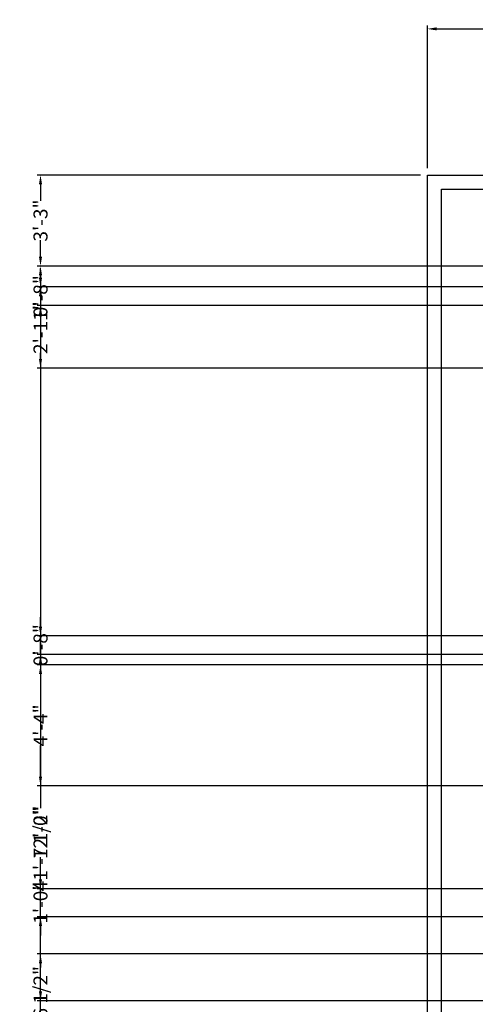
# Model space of a CAD drawing. Units: inches. Extents: x 6704 to 7574, y 11759 to 12617.
# Tile 3 of 8: x 6704 to 6900, y 12195 to 12617. Entities that reach past the tile are written whole.
import ezdxf

# ---------------------------------------------------------------- set-up
doc = ezdxf.new("R2010")
doc.units = ezdxf.units.IN
doc.header["$MEASUREMENT"] = 0
doc.layers.add('C-PROP', color=7, linetype='Continuous', lineweight=30)
doc.layers.add('YQ_DIM', color=3, linetype='Continuous', lineweight=18)
doc.styles.get("Standard").update_dxf_attribs({"font": 'arial.ttf'})
doc.dimstyles.new('yqi0', dxfattribs={"dimscale": 0, "dimtxt": 6, "dimasz": 4, "dimexe": 1.5, "dimexo": 3, "dimgap": 0.5, "dimtad": 0, "dimdsep": 46, "dimlunit": 4, "dimtxsty": 'Standard', "dimcen": 0, "dimclrd": 256, "dimclre": 256, "dimclrt": 7, "dimadec": 1, "dimazin": 2, "dimtfac": 1, "dimtix": 1, "dimtmove": 2, "dimatfit": 2, "dimfxl": 1, "dimtolj": 1, "dimtzin": 0, "dimarcsym": 0})

# ---------------------------------------------------------------- blocks, each defined once
blk = doc.blocks.new('*D2')
at = {"layer": 'Defpoints', "color": 0, "transparency": 16777216}
for p in [(7311.07, 12612.93), (6879.07, 12550.26), (7311.07, 12550.26)]:
    blk.add_point(p, dxfattribs=at)
at = {"layer": 'YQ_DIM', "color": 0, "lineweight": -2, "transparency": 16777216}
for p, q in [((6879.07, 12553.26), (6879.07, 12614.43)), ((7311.07, 12553.26), (7311.07, 12614.43)), ((6883.07, 12612.93), (7089.48, 12612.93)), ((7307.07, 12612.93), (7100.66, 12612.93))]:
    blk.add_line(p, q, dxfattribs=at)
at = {"layer": 'YQ_DIM', "color": 0, "transparency": 16777216}
for points in [[(6883.07, 12613.6), (6883.07, 12612.27), (6879.07, 12612.93)], [(7307.07, 12613.6), (7307.07, 12612.27), (7311.07, 12612.93)]]:
    blk.add_solid(points, dxfattribs=at)
at = {"layer": 'YQ_DIM', "color": 0, "transparency": 16777216, "insert": (7095.07, 12612.93), "char_height": 6, "attachment_point": 5}
blk.add_mtext("\\A1;36'", dxfattribs=at)
blk = doc.blocks.new('*D56')
at = {"layer": 'Defpoints', "color": 0, "transparency": 16777216}
for p in [(6712.97, 12511.26), (6918.07, 12511.26), (6918.07, 12011.76)]:
    blk.add_point(p, dxfattribs=at)
at = {"layer": 'YQ_DIM', "lineweight": -2, "transparency": 16777216}
for p, q in [((6915.07, 12511.26), (6711.47, 12511.26)), ((6712.97, 12507.26), (6712.97, 12279.42)), ((6712.97, 12015.76), (6712.97, 12243.59)), ((6915.07, 12011.76), (6711.47, 12011.76))]:
    blk.add_line(p, q, dxfattribs=at)
at = {"layer": 'YQ_DIM', "transparency": 16777216}
for points in [[(6712.3, 12507.26), (6713.64, 12507.26), (6712.97, 12511.26)], [(6712.3, 12015.76), (6713.64, 12015.76), (6712.97, 12011.76)]]:
    blk.add_solid(points, dxfattribs=at)
at = {"layer": 'YQ_DIM', "color": 7, "transparency": 16777216, "insert": (6712.97, 12261.51), "char_height": 6, "attachment_point": 5, "rotation": 90}
blk.add_mtext('\\A1;41\'-7 1/2"', dxfattribs=at)
blk = doc.blocks.new('*D57')
at = {"layer": 'Defpoints', "color": 0, "transparency": 16777216}
for p in [(6879.07, 12550.26), (6712.97, 12511.26), (6918.07, 12511.26)]:
    blk.add_point(p, dxfattribs=at)
at = {"layer": 'YQ_DIM', "lineweight": -2, "transparency": 16777216}
for p, q in [((6876.07, 12550.26), (6711.47, 12550.26)), ((6712.97, 12546.26), (6712.97, 12539.23)), ((6712.97, 12515.26), (6712.97, 12522.28)), ((6915.07, 12511.26), (6711.47, 12511.26))]:
    blk.add_line(p, q, dxfattribs=at)
at = {"layer": 'YQ_DIM', "transparency": 16777216}
for points in [[(6712.3, 12546.26), (6713.64, 12546.26), (6712.97, 12550.26)], [(6712.3, 12515.26), (6713.64, 12515.26), (6712.97, 12511.26)]]:
    blk.add_solid(points, dxfattribs=at)
at = {"layer": 'YQ_DIM', "color": 7, "transparency": 16777216, "insert": (6712.97, 12530.76), "char_height": 6, "attachment_point": 5, "rotation": 90}
blk.add_mtext('\\A1;3\'-3"', dxfattribs=at)
blk = doc.blocks.new('*D67')
at = {"layer": 'Defpoints', "color": 0, "transparency": 16777216}
for p in [(6712.97, 12340.26), (6927.07, 12340.26), (6927.07, 12196.26)]:
    blk.add_point(p, dxfattribs=at)
at = {"layer": 'YQ_DIM', "lineweight": -2, "transparency": 16777216}
for p, q in [((6924.07, 12340.26), (6711.47, 12340.26)), ((6712.97, 12336.26), (6712.97, 12278.78)), ((6712.97, 12200.26), (6712.97, 12257.73)), ((6924.07, 12196.26), (6711.47, 12196.26))]:
    blk.add_line(p, q, dxfattribs=at)
at = {"layer": 'YQ_DIM', "transparency": 16777216}
for points in [[(6712.3, 12336.26), (6713.64, 12336.26), (6712.97, 12340.26)], [(6712.3, 12200.26), (6713.64, 12200.26), (6712.97, 12196.26)]]:
    blk.add_solid(points, dxfattribs=at)
at = {"layer": 'YQ_DIM', "color": 7, "transparency": 16777216, "insert": (6712.97, 12268.26), "char_height": 6, "attachment_point": 5, "rotation": 90}
blk.add_mtext('\\A1;12\'-0"', dxfattribs=at)
blk = doc.blocks.new('*D76')
at = {"layer": 'Defpoints', "color": 0, "transparency": 16777216}
for p in [(7260.07, 12502.26), (6712.97, 12467.43), (7260.07, 12467.43)]:
    blk.add_point(p, dxfattribs=at)
at = {"layer": 'YQ_DIM', "lineweight": -2, "transparency": 16777216}
for p, q in [((7257.07, 12502.26), (6711.47, 12502.26)), ((6712.97, 12498.26), (6712.97, 12495.7)), ((6712.97, 12471.43), (6712.97, 12473.99)), ((7257.07, 12467.43), (6711.47, 12467.43))]:
    blk.add_line(p, q, dxfattribs=at)
at = {"layer": 'YQ_DIM', "transparency": 16777216}
for points in [[(6712.3, 12498.26), (6713.64, 12498.26), (6712.97, 12502.26)], [(6712.3, 12471.43), (6713.64, 12471.43), (6712.97, 12467.43)]]:
    blk.add_solid(points, dxfattribs=at)
at = {"layer": 'YQ_DIM', "color": 7, "transparency": 16777216, "insert": (6712.97, 12484.84), "char_height": 6, "attachment_point": 5, "rotation": 90}
blk.add_mtext('\\A1;2\'-11"', dxfattribs=at)
blk = doc.blocks.new('*D77')
at = {"layer": 'Defpoints', "color": 0, "transparency": 16777216}
for p in [(7260.07, 12216.3), (6712.97, 12173.76), (7260.07, 12173.76)]:
    blk.add_point(p, dxfattribs=at)
at = {"layer": 'YQ_DIM', "lineweight": -2, "transparency": 16777216}
for p, q in [((7257.07, 12216.3), (6711.47, 12216.3)), ((6712.97, 12212.3), (6712.97, 12210.49)), ((6712.97, 12177.76), (6712.97, 12179.57)), ((7257.07, 12173.76), (6711.47, 12173.76))]:
    blk.add_line(p, q, dxfattribs=at)
at = {"layer": 'YQ_DIM', "transparency": 16777216}
for points in [[(6712.3, 12212.3), (6713.64, 12212.3), (6712.97, 12216.3)], [(6712.3, 12177.76), (6713.64, 12177.76), (6712.97, 12173.76)]]:
    blk.add_solid(points, dxfattribs=at)
at = {"layer": 'YQ_DIM', "color": 7, "transparency": 16777216, "insert": (6712.97, 12195.03), "char_height": 6, "attachment_point": 5, "rotation": 90}
blk.add_mtext('\\A1;3\'-6 1/2"', dxfattribs=at)
blk = doc.blocks.new('*D78')
at = {"layer": 'Defpoints', "color": 0, "transparency": 16777216}
for p in [(6712.97, 12352.63), (6927.07, 12352.63), (6927.07, 12344.76)]:
    blk.add_point(p, dxfattribs=at)
at = {"layer": 'YQ_DIM', "lineweight": -2, "transparency": 16777216}
for p, q in [((6712.97, 12356.63), (6712.97, 12360.63)), ((6924.07, 12352.63), (6711.47, 12352.63)), ((6712.97, 12344.76), (6712.97, 12352.63)), ((6924.07, 12344.76), (6711.47, 12344.76)), ((6712.97, 12340.76), (6712.97, 12336.76))]:
    blk.add_line(p, q, dxfattribs=at)
at = {"layer": 'YQ_DIM', "transparency": 16777216}
for points in [[(6712.3, 12356.63), (6713.64, 12356.63), (6712.97, 12352.63)], [(6712.3, 12340.76), (6713.64, 12340.76), (6712.97, 12344.76)]]:
    blk.add_solid(points, dxfattribs=at)
at = {"layer": 'YQ_DIM', "color": 7, "transparency": 16777216, "insert": (6712.97, 12348.69), "char_height": 6, "attachment_point": 5, "rotation": 90}
blk.add_mtext('\\A1;0\'-8"', dxfattribs=at)
blk = doc.blocks.new('*D81')
at = {"layer": 'Defpoints', "color": 0, "transparency": 16777216}
for p in [(7063.57, 12502.26), (6712.97, 12494.38), (7063.57, 12494.38)]:
    blk.add_point(p, dxfattribs=at)
at = {"layer": 'YQ_DIM', "lineweight": -2, "transparency": 16777216}
for p, q in [((6712.97, 12506.26), (6712.97, 12510.26)), ((7060.57, 12502.26), (6711.47, 12502.26)), ((6712.97, 12502.26), (6712.97, 12494.38)), ((7060.57, 12494.38), (6711.47, 12494.38)), ((6712.97, 12490.38), (6712.97, 12486.38))]:
    blk.add_line(p, q, dxfattribs=at)
at = {"layer": 'YQ_DIM', "transparency": 16777216}
for points in [[(6712.3, 12506.26), (6713.64, 12506.26), (6712.97, 12502.26)], [(6712.3, 12490.38), (6713.64, 12490.38), (6712.97, 12494.38)]]:
    blk.add_solid(points, dxfattribs=at)
at = {"layer": 'YQ_DIM', "color": 7, "transparency": 16777216, "insert": (6712.97, 12498.32), "char_height": 6, "attachment_point": 5, "rotation": 90}
blk.add_mtext('\\A1;0\'-8"', dxfattribs=at)
blk = doc.blocks.new('*D86')
at = {"layer": 'Defpoints', "color": 0, "transparency": 16777216}
for p in [(6712.97, 12340.26), (6927.07, 12340.26), (6927.07, 12288.32)]:
    blk.add_point(p, dxfattribs=at)
at = {"layer": 'YQ_DIM', "lineweight": -2, "transparency": 16777216}
for p, q in [((6924.07, 12340.26), (6711.47, 12340.26)), ((6712.97, 12336.26), (6712.97, 12322.88)), ((6712.97, 12292.32), (6712.97, 12305.69)), ((6924.07, 12288.32), (6711.47, 12288.32))]:
    blk.add_line(p, q, dxfattribs=at)
at = {"layer": 'YQ_DIM', "transparency": 16777216}
for points in [[(6712.3, 12336.26), (6713.64, 12336.26), (6712.97, 12340.26)], [(6712.3, 12292.32), (6713.64, 12292.32), (6712.97, 12288.32)]]:
    blk.add_solid(points, dxfattribs=at)
at = {"layer": 'YQ_DIM', "color": 7, "transparency": 16777216, "insert": (6712.97, 12314.29), "char_height": 6, "attachment_point": 5, "rotation": 90}
blk.add_mtext('\\A1;4\'-4"', dxfattribs=at)
blk = doc.blocks.new('*D87')
at = {"layer": 'Defpoints', "color": 0, "transparency": 16777216}
for p in [(6712.97, 12244.26), (6927.07, 12244.26), (6927.07, 12232.26)]:
    blk.add_point(p, dxfattribs=at)
at = {"layer": 'YQ_DIM', "lineweight": -2, "transparency": 16777216}
for p, q in [((6712.97, 12248.26), (6712.97, 12252.26)), ((6924.07, 12244.26), (6711.47, 12244.26)), ((6712.97, 12232.26), (6712.97, 12244.26)), ((6924.07, 12232.26), (6711.47, 12232.26)), ((6712.97, 12228.26), (6712.97, 12224.26))]:
    blk.add_line(p, q, dxfattribs=at)
at = {"layer": 'YQ_DIM', "transparency": 16777216}
for points in [[(6712.3, 12248.26), (6713.64, 12248.26), (6712.97, 12244.26)], [(6712.3, 12228.26), (6713.64, 12228.26), (6712.97, 12232.26)]]:
    blk.add_solid(points, dxfattribs=at)
at = {"layer": 'YQ_DIM', "color": 7, "transparency": 16777216, "insert": (6712.97, 12238.26), "char_height": 6, "attachment_point": 5, "rotation": 90}
blk.add_mtext('\\A1;1\'-0"', dxfattribs=at)

msp = doc.modelspace()

# ---------------------------------------------------------------- linework, layer by layer
at = {"layer": 'C-PROP'}
for p, q in [((6879.073, 11951.757), (6879.073, 12550.257)), ((6879.073, 12550.257), (7311.073, 12550.257)), ((6885.073, 12544.257), (7305.073, 12544.257)), ((6885.073, 11957.757), (6885.073, 12544.257))]:
    msp.add_line(p, q, dxfattribs=at)

# ---------------------------------------------------------------- dimensions: what is measured, and where the dimension line sits
at = {"layer": 'YQ_DIM'}
dim = msp.add_aligned_dim(p1=(6879.073, 12550.257), p2=(7311.073, 12550.257), distance=62.676, dimstyle='yqi0', override={"dimscale": 1, "dimclrd": 0, "dimclre": 0, "dimclrt": 0}, dxfattribs=at)
dim.commit()
dim.dimension.update_dxf_attribs({"geometry": '*D2', "text_midpoint": (7095.073, 12612.934)})
for base, p1, p2, picture, middle in [((6712.97, 12511.257), (6879.073, 12550.257), (6918.073, 12511.257), '*D57', (6712.97, 12530.757)), ((6712.97, 12511.257), (6918.073, 12011.757), (6918.073, 12511.257), '*D56', (6712.97, 12261.507)), ((6712.97, 12494.383), (7063.573, 12502.257), (7063.573, 12494.383), '*D81', (6712.97, 12498.32)), ((6712.97, 12467.428), (7260.073, 12502.257), (7260.073, 12467.428), '*D76', (6712.97, 12484.842)), ((6712.97, 12352.631), (6927.073, 12344.757), (6927.073, 12352.631), '*D78', (6712.97, 12348.694)), ((6712.97, 12340.257), (6927.073, 12196.257), (6927.073, 12340.257), '*D67', (6712.97, 12268.257)), ((6712.97, 12340.257), (6927.073, 12288.32), (6927.073, 12340.257), '*D86', (6712.97, 12314.289)), ((6712.97, 12244.257), (6927.073, 12232.257), (6927.073, 12244.257), '*D87', (6712.97, 12238.257)), ((6712.97, 12173.757), (7260.073, 12216.302), (7260.073, 12173.757), '*D77', (6712.97, 12195.029))]:
    dim = msp.add_linear_dim(base=base, p1=p1, p2=p2, angle=90, dimstyle='yqi0', override={"dimscale": 1, "dimdec": 1, "dimzin": 1, "dimfrac": 2}, dxfattribs=at)
    dim.commit()
    dim.dimension.update_dxf_attribs({"geometry": picture, "text_midpoint": middle})

doc.saveas('drawing.dxf')
